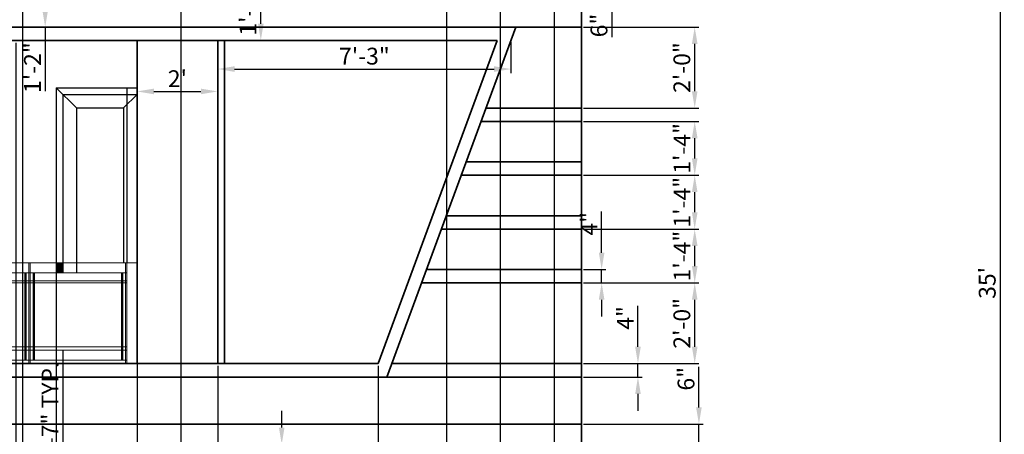
# Model space of a CAD drawing. Units: inches. Extents: x 2406 to 2953, y 1777 to 2285.
# Tile 4 of 5: x 2661 to 2953, y 1987 to 2111. Entities that reach past the tile are written whole.
import ezdxf

# ---------------------------------------------------------------- set-up
doc = ezdxf.new("R2010")
doc.units = ezdxf.units.IN
for name, color, linetype, lineweight in [('A-ANNO-DIMS', 2, 'Continuous', 18), ('A-ELEV', 7, 'Continuous', 35), ('A-ELEV-PATT', 253, 'Continuous', 13), ('A-FLOR-HRAL', 6, 'Continuous', 18), ('A-GLAZ', 4, 'Continuous', 25)]:
    doc.layers.add(name, color=color, linetype=linetype, lineweight=lineweight)
doc.styles.get("Standard").update_dxf_attribs({"font": 'arial.ttf'})
doc.dimstyles.new('ISO-25', dxfattribs={"dimtxt": 5, "dimasz": 5, "dimexe": 1.25, "dimexo": 0.625, "dimtad": 1, "dimdec": 0, "dimlunit": 3, "dimtxsty": 'Standard', "dimcen": 2.5, "dimadec": 0, "dimazin": 0, "dimtfac": 1, "dimtdec": 0, "dimtmove": 0, "dimatfit": 3, "dimfxl": 1, "dimarcsym": 0})

# ---------------------------------------------------------------- blocks, each defined once
blk = doc.blocks.new('*D1')
at = {"layer": 'A-ANNO-DIMS', "color": 0, "lineweight": -2, "transparency": 16777216}
for p, q in [((2828.46, 2242.34), (2953.44, 2242.34)), ((2952.19, 2237.34), (2952.19, 1827.34)), ((2828.46, 1822.34), (2953.44, 1822.34))]:
    blk.add_line(p, q, dxfattribs=at)
at = {"layer": 'A-ANNO-DIMS', "color": 0, "transparency": 16777216}
for points in [[(2951.35, 2237.34), (2953.02, 2237.34), (2952.19, 2242.34)], [(2951.35, 1827.34), (2953.02, 1827.34), (2952.19, 1822.34)]]:
    blk.add_solid(points, dxfattribs=at)
at = {"layer": 'Defpoints', "color": 0, "transparency": 16777216}
for p in [(2827.83, 2242.34), (2827.83, 1822.34), (2952.19, 1822.34)]:
    blk.add_point(p, dxfattribs=at)
at = {"layer": 'A-ANNO-DIMS', "color": 0, "transparency": 16777216, "insert": (2949.01, 2032.34), "char_height": 5, "attachment_point": 5, "rotation": 90}
blk.add_mtext("35'", dxfattribs=at)
blk = doc.blocks.new('*D4')
at = {"layer": 'A-ANNO-DIMS', "color": 0, "lineweight": -2, "transparency": 16777216}
for p, q in [((2719.83, 2103.72), (2719.83, 2094.64)), ((2806.9, 2103.89), (2806.9, 2094.64)), ((2724.83, 2095.89), (2801.9, 2095.89))]:
    blk.add_line(p, q, dxfattribs=at)
at = {"layer": 'A-ANNO-DIMS', "color": 0, "transparency": 16777216}
for points in [[(2724.83, 2096.72), (2724.83, 2095.05), (2719.83, 2095.89)], [(2801.9, 2096.72), (2801.9, 2095.05), (2806.9, 2095.89)]]:
    blk.add_solid(points, dxfattribs=at)
at = {"layer": 'Defpoints', "color": 0, "transparency": 16777216}
for p in [(2719.83, 2104.34), (2806.9, 2104.52), (2806.9, 2095.89)]:
    blk.add_point(p, dxfattribs=at)
at = {"layer": 'A-ANNO-DIMS', "color": 0, "transparency": 16777216, "insert": (2763.37, 2099.07), "char_height": 5, "attachment_point": 5}
blk.add_mtext('7\'-3"', dxfattribs=at)
blk = doc.blocks.new('*D19')
at = {"layer": 'A-ANNO-DIMS', "color": 0, "lineweight": -2, "transparency": 16777216}
for p, q in [((2862.73, 1995.34), (2862.73, 2007.37)), ((2828.46, 1990.34), (2863.98, 1990.34)), ((2862.73, 1984.34), (2862.73, 1990.34)), ((2828.46, 1984.34), (2863.98, 1984.34)), ((2862.73, 1979.34), (2862.73, 1974.34))]:
    blk.add_line(p, q, dxfattribs=at)
at = {"layer": 'A-ANNO-DIMS', "color": 0, "transparency": 16777216}
for points in [[(2861.89, 1995.34), (2863.56, 1995.34), (2862.73, 1990.34)], [(2861.89, 1979.34), (2863.56, 1979.34), (2862.73, 1984.34)]]:
    blk.add_solid(points, dxfattribs=at)
at = {"layer": 'Defpoints', "color": 0, "transparency": 16777216}
for p in [(2827.83, 1990.34), (2862.73, 1990.34), (2827.83, 1984.34)]:
    blk.add_point(p, dxfattribs=at)
at = {"layer": 'A-ANNO-DIMS', "color": 0, "transparency": 16777216, "insert": (2859.55, 2003.85), "char_height": 5, "attachment_point": 5, "rotation": 90}
blk.add_mtext('6"', dxfattribs=at)
blk = doc.blocks.new('*D20')
at = {"layer": 'A-ANNO-DIMS', "color": 0, "lineweight": -2, "transparency": 16777216}
for p, q in [((2844.62, 2013.34), (2844.62, 2025.54)), ((2828.46, 2008.34), (2845.87, 2008.34)), ((2844.62, 2004.34), (2844.62, 2008.34)), ((2828.46, 2004.34), (2845.87, 2004.34)), ((2844.62, 1999.34), (2844.62, 1994.34))]:
    blk.add_line(p, q, dxfattribs=at)
at = {"layer": 'A-ANNO-DIMS', "color": 0, "transparency": 16777216}
for points in [[(2843.79, 2013.34), (2845.46, 2013.34), (2844.62, 2008.34)], [(2843.79, 1999.34), (2845.46, 1999.34), (2844.62, 2004.34)]]:
    blk.add_solid(points, dxfattribs=at)
at = {"layer": 'Defpoints', "color": 0, "transparency": 16777216}
for p in [(2827.83, 2008.34), (2844.62, 2008.34), (2827.83, 2004.34)]:
    blk.add_point(p, dxfattribs=at)
at = {"layer": 'A-ANNO-DIMS', "color": 0, "transparency": 16777216, "insert": (2841.5, 2021.94), "char_height": 5, "attachment_point": 5, "rotation": 90}
blk.add_mtext('4"', dxfattribs=at)
blk = doc.blocks.new('*D21')
at = {"layer": 'A-ANNO-DIMS', "color": 0, "lineweight": -2, "transparency": 16777216}
for p, q in [((2833.84, 2041.31), (2833.84, 2053.51)), ((2828.46, 2036.31), (2835.09, 2036.31)), ((2833.84, 2032.31), (2833.84, 2036.31)), ((2828.46, 2032.31), (2835.09, 2032.31)), ((2833.84, 2027.31), (2833.84, 2022.31))]:
    blk.add_line(p, q, dxfattribs=at)
at = {"layer": 'A-ANNO-DIMS', "color": 0, "transparency": 16777216}
for points in [[(2833, 2041.31), (2834.67, 2041.31), (2833.84, 2036.31)], [(2833, 2027.31), (2834.67, 2027.31), (2833.84, 2032.31)]]:
    blk.add_solid(points, dxfattribs=at)
at = {"layer": 'Defpoints', "color": 0, "transparency": 16777216}
for p in [(2827.83, 2036.31), (2833.84, 2036.31), (2827.83, 2032.31)]:
    blk.add_point(p, dxfattribs=at)
at = {"layer": 'A-ANNO-DIMS', "color": 0, "transparency": 16777216, "insert": (2830.71, 2049.91), "char_height": 5, "attachment_point": 5, "rotation": 90}
blk.add_mtext('4"', dxfattribs=at)
blk = doc.blocks.new('*D25')
at = {"layer": 'A-ANNO-DIMS', "color": 0, "lineweight": -2, "transparency": 16777216}
for p, q in [((2695.83, 2094.79), (2695.83, 2087.98)), ((2719.83, 2095.26), (2719.83, 2087.98)), ((2700.83, 2089.23), (2714.83, 2089.23))]:
    blk.add_line(p, q, dxfattribs=at)
at = {"layer": 'A-ANNO-DIMS', "color": 0, "transparency": 16777216}
for points in [[(2700.83, 2090.06), (2700.83, 2088.4), (2695.83, 2089.23)], [(2714.83, 2090.06), (2714.83, 2088.4), (2719.83, 2089.23)]]:
    blk.add_solid(points, dxfattribs=at)
at = {"layer": 'Defpoints', "color": 0, "transparency": 16777216}
for p in [(2695.83, 2095.42), (2719.83, 2095.89), (2719.83, 2089.23)]:
    blk.add_point(p, dxfattribs=at)
at = {"layer": 'A-ANNO-DIMS', "color": 0, "transparency": 16777216, "insert": (2707.83, 2092.37), "char_height": 5, "attachment_point": 5}
blk.add_mtext("2'", dxfattribs=at)
blk = doc.blocks.new('*D26')
at = {"layer": 'A-ANNO-DIMS', "color": 0, "lineweight": -2, "transparency": 16777216}
for p, q in [((2680.71, 2122.34), (2667.31, 2122.34)), ((2668.56, 2117.34), (2668.56, 2113.34)), ((2680.71, 2108.34), (2667.31, 2108.34)), ((2668.56, 2108.34), (2668.56, 2089.27))]:
    blk.add_line(p, q, dxfattribs=at)
at = {"layer": 'A-ANNO-DIMS', "color": 0, "transparency": 16777216}
for points in [[(2667.73, 2117.34), (2669.4, 2117.34), (2668.56, 2122.34)], [(2667.73, 2113.34), (2669.4, 2113.34), (2668.56, 2108.34)]]:
    blk.add_solid(points, dxfattribs=at)
at = {"layer": 'Defpoints', "color": 0, "transparency": 16777216}
for p in [(2681.33, 2122.34), (2668.56, 2108.34), (2681.33, 2108.34)]:
    blk.add_point(p, dxfattribs=at)
at = {"layer": 'A-ANNO-DIMS', "color": 0, "transparency": 16777216, "insert": (2665.43, 2096.31), "char_height": 5, "attachment_point": 5, "rotation": 90}
blk.add_mtext('1\'-2"', dxfattribs=at)
blk = doc.blocks.new('*D27')
at = {"layer": 'A-ANNO-DIMS', "color": 0, "lineweight": -2, "transparency": 16777216}
for p, q in [((2737.53, 2122.34), (2731.35, 2122.34)), ((2732.6, 2109.34), (2732.6, 2117.34)), ((2737.53, 2104.34), (2731.35, 2104.34))]:
    blk.add_line(p, q, dxfattribs=at)
at = {"layer": 'A-ANNO-DIMS', "color": 0, "transparency": 16777216}
for points in [[(2731.77, 2117.34), (2733.44, 2117.34), (2732.6, 2122.34)], [(2731.77, 2109.34), (2733.44, 2109.34), (2732.6, 2104.34)]]:
    blk.add_solid(points, dxfattribs=at)
at = {"layer": 'Defpoints', "color": 0, "transparency": 16777216}
for p in [(2732.6, 2122.34), (2738.16, 2122.34), (2738.16, 2104.34)]:
    blk.add_point(p, dxfattribs=at)
at = {"layer": 'A-ANNO-DIMS', "color": 0, "transparency": 16777216, "insert": (2729.43, 2113.34), "char_height": 5, "attachment_point": 5, "rotation": 90}
blk.add_mtext('1\'-6"', dxfattribs=at)
blk = doc.blocks.new('*D29')
at = {"layer": 'A-ANNO-DIMS', "color": 0, "lineweight": -2, "transparency": 16777216}
for p, q in [((2836.87, 2133.34), (2836.87, 2138.34)), ((2828.46, 2128.34), (2838.12, 2128.34)), ((2836.87, 2128.34), (2836.87, 2122.34)), ((2828.46, 2122.34), (2838.12, 2122.34)), ((2836.87, 2117.34), (2836.87, 2105.32))]:
    blk.add_line(p, q, dxfattribs=at)
at = {"layer": 'A-ANNO-DIMS', "color": 0, "transparency": 16777216}
for points in [[(2836.03, 2133.34), (2837.7, 2133.34), (2836.87, 2128.34)], [(2836.03, 2117.34), (2837.7, 2117.34), (2836.87, 2122.34)]]:
    blk.add_solid(points, dxfattribs=at)
at = {"layer": 'Defpoints', "color": 0, "transparency": 16777216}
for p in [(2827.83, 2128.34), (2827.83, 2122.34), (2836.87, 2122.34)]:
    blk.add_point(p, dxfattribs=at)
at = {"layer": 'A-ANNO-DIMS', "color": 0, "transparency": 16777216, "insert": (2833.69, 2108.83), "char_height": 5, "attachment_point": 5, "rotation": 90}
blk.add_mtext('6"', dxfattribs=at)
blk = doc.blocks.new('*D32')
at = {"layer": 'A-ANNO-DIMS', "color": 0, "lineweight": -2, "transparency": 16777216}
for p, q in [((2738.81, 1989.34), (2738.81, 1994.34)), ((2748.35, 1984.34), (2737.56, 1984.34)), ((2738.81, 1975.34), (2738.81, 1984.34)), ((2748.35, 1975.34), (2737.56, 1975.34)), ((2738.81, 1970.34), (2738.81, 1965.34))]:
    blk.add_line(p, q, dxfattribs=at)
at = {"layer": 'A-ANNO-DIMS', "color": 0, "transparency": 16777216}
for points in [[(2737.98, 1989.34), (2739.65, 1989.34), (2738.81, 1984.34)], [(2737.98, 1970.34), (2739.65, 1970.34), (2738.81, 1975.34)]]:
    blk.add_solid(points, dxfattribs=at)
at = {"layer": 'Defpoints', "color": 0, "transparency": 16777216}
for p in [(2738.81, 1984.34), (2748.98, 1984.34), (2748.98, 1975.34)]:
    blk.add_point(p, dxfattribs=at)
at = {"layer": 'A-ANNO-DIMS', "color": 0, "transparency": 16777216, "insert": (2735.64, 1979.84), "char_height": 5, "attachment_point": 5, "rotation": 90}
blk.add_mtext('9"', dxfattribs=at)
blk = doc.blocks.new('*D45')
at = {"layer": 'A-ANNO-DIMS', "color": 0, "lineweight": -2, "transparency": 16777216}
for p, q in [((2673.85, 1912.9), (2673.85, 2012.41)), ((2681.47, 1912.9), (2672.6, 1912.9)), ((2673.85, 1862.91), (2673.85, 1907.9)), ((2681.47, 1857.91), (2672.6, 1857.91))]:
    blk.add_line(p, q, dxfattribs=at)
at = {"layer": 'A-ANNO-DIMS', "color": 0, "transparency": 16777216}
for points in [[(2673.01, 1907.9), (2674.68, 1907.9), (2673.85, 1912.9)], [(2673.01, 1862.91), (2674.68, 1862.91), (2673.85, 1857.91)]]:
    blk.add_solid(points, dxfattribs=at)
at = {"layer": 'Defpoints', "color": 0, "transparency": 16777216}
for p in [(2673.85, 1912.9), (2682.1, 1912.9), (2682.1, 1857.91)]:
    blk.add_point(p, dxfattribs=at)
at = {"layer": 'A-ANNO-DIMS', "color": 0, "transparency": 16777216, "insert": (2670.64, 1965.16), "char_height": 5, "attachment_point": 5, "rotation": 90}
blk.add_mtext('GATE ORNAMENT 4\'-7" TYP.', dxfattribs=at)
blk = doc.blocks.new('*D51')
at = {"layer": 'A-ANNO-DIMS', "color": 0, "lineweight": -2, "transparency": 16777216}
for p, q in [((2787.83, 1984.97), (2787.83, 2275.24)), ((2792.83, 2273.99), (2798.83, 2273.99)), ((2803.83, 1984.97), (2803.83, 2275.24))]:
    blk.add_line(p, q, dxfattribs=at)
at = {"layer": 'A-ANNO-DIMS', "color": 0, "transparency": 16777216}
for points in [[(2792.83, 2274.82), (2792.83, 2273.16), (2787.83, 2273.99)], [(2798.83, 2274.82), (2798.83, 2273.16), (2803.83, 2273.99)]]:
    blk.add_solid(points, dxfattribs=at)
at = {"layer": 'Defpoints', "color": 0, "transparency": 16777216}
for p in [(2803.83, 2273.99), (2787.83, 1984.34), (2803.83, 1984.34)]:
    blk.add_point(p, dxfattribs=at)
at = {"layer": 'A-ANNO-DIMS', "color": 0, "transparency": 16777216, "insert": (2795.83, 2277.13), "char_height": 5, "attachment_point": 5}
blk.add_mtext('1\'-4"', dxfattribs=at)
blk = doc.blocks.new('*D52')
at = {"layer": 'A-ANNO-DIMS', "color": 0, "lineweight": -2, "transparency": 16777216}
for p, q in [((2803.83, 1984.97), (2803.83, 2275.24)), ((2808.83, 2273.99), (2814.83, 2273.99)), ((2819.83, 1984.97), (2819.83, 2275.24))]:
    blk.add_line(p, q, dxfattribs=at)
at = {"layer": 'A-ANNO-DIMS', "color": 0, "transparency": 16777216}
for points in [[(2808.83, 2274.82), (2808.83, 2273.16), (2803.83, 2273.99)], [(2814.83, 2274.82), (2814.83, 2273.16), (2819.83, 2273.99)]]:
    blk.add_solid(points, dxfattribs=at)
at = {"layer": 'Defpoints', "color": 0, "transparency": 16777216}
for p in [(2819.83, 2273.99), (2803.83, 1984.34), (2819.83, 1984.34)]:
    blk.add_point(p, dxfattribs=at)
at = {"layer": 'A-ANNO-DIMS', "color": 0, "transparency": 16777216, "insert": (2811.83, 2277.13), "char_height": 5, "attachment_point": 5}
blk.add_mtext('1\'-4"', dxfattribs=at)
blk = doc.blocks.new('*D53')
at = {"layer": 'A-ANNO-DIMS', "color": 0, "lineweight": -2, "transparency": 16777216}
for p, q in [((2814.83, 2273.99), (2809.83, 2273.99)), ((2819.83, 1984.97), (2819.83, 2275.24)), ((2819.83, 2273.99), (2827.83, 2273.99)), ((2827.83, 1984.97), (2827.83, 2275.24)), ((2832.83, 2273.99), (2852.37, 2273.99))]:
    blk.add_line(p, q, dxfattribs=at)
at = {"layer": 'A-ANNO-DIMS', "color": 0, "transparency": 16777216}
for points in [[(2814.83, 2274.82), (2814.83, 2273.16), (2819.83, 2273.99)], [(2832.83, 2274.82), (2832.83, 2273.16), (2827.83, 2273.99)]]:
    blk.add_solid(points, dxfattribs=at)
at = {"layer": 'Defpoints', "color": 0, "transparency": 16777216}
for p in [(2827.83, 2273.99), (2819.83, 1984.34), (2827.83, 1984.34)]:
    blk.add_point(p, dxfattribs=at)
at = {"layer": 'A-ANNO-DIMS', "color": 0, "transparency": 16777216, "insert": (2845.1, 2277.17), "char_height": 5, "attachment_point": 5}
blk.add_mtext('0\'-8"', dxfattribs=at)
blk = doc.blocks.new('*D64')
at = {"layer": 'A-ANNO-DIMS', "color": 0, "lineweight": -2, "transparency": 16777216}
for p, q in [((2659.83, 2103.72), (2659.83, 1793.44)), ((2671.83, 2089.72), (2671.83, 1793.44)), ((2664.83, 1794.69), (2666.83, 1794.69)), ((2671.83, 1794.69), (2690.9, 1794.69))]:
    blk.add_line(p, q, dxfattribs=at)
at = {"layer": 'A-ANNO-DIMS', "color": 0, "transparency": 16777216}
for points in [[(2664.83, 1795.52), (2664.83, 1793.86), (2659.83, 1794.69)], [(2666.83, 1795.52), (2666.83, 1793.86), (2671.83, 1794.69)]]:
    blk.add_solid(points, dxfattribs=at)
at = {"layer": 'Defpoints', "color": 0, "transparency": 16777216}
for p in [(2659.83, 2104.34), (2671.83, 2090.34), (2671.83, 1794.69)]:
    blk.add_point(p, dxfattribs=at)
at = {"layer": 'A-ANNO-DIMS', "color": 0, "transparency": 16777216, "insert": (2683.87, 1797.87), "char_height": 5, "attachment_point": 5}
blk.add_mtext('1\'-0"', dxfattribs=at)
blk = doc.blocks.new('*D65')
at = {"layer": 'A-ANNO-DIMS', "color": 0, "lineweight": -2, "transparency": 16777216}
for p, q in [((2671.83, 2089.72), (2671.83, 1793.44)), ((2695.83, 2089.72), (2695.83, 1793.44)), ((2676.83, 1794.69), (2690.83, 1794.69))]:
    blk.add_line(p, q, dxfattribs=at)
at = {"layer": 'A-ANNO-DIMS', "color": 0, "transparency": 16777216}
for points in [[(2676.83, 1795.52), (2676.83, 1793.86), (2671.83, 1794.69)], [(2690.83, 1795.52), (2690.83, 1793.86), (2695.83, 1794.69)]]:
    blk.add_solid(points, dxfattribs=at)
at = {"layer": 'Defpoints', "color": 0, "transparency": 16777216}
for p in [(2671.83, 2090.34), (2695.83, 2090.34), (2695.83, 1794.69)]:
    blk.add_point(p, dxfattribs=at)
at = {"layer": 'A-ANNO-DIMS', "color": 0, "transparency": 16777216, "insert": (2683.83, 1797.87), "char_height": 5, "attachment_point": 5}
blk.add_mtext('2\'-0"', dxfattribs=at)
blk = doc.blocks.new('*D67')
at = {"layer": 'A-ANNO-DIMS', "color": 0, "lineweight": -2, "transparency": 16777216}
for p, q in [((2719.83, 2007.72), (2719.83, 1793.44)), ((2767.46, 2007.72), (2767.46, 1793.44)), ((2724.83, 1794.69), (2762.46, 1794.69))]:
    blk.add_line(p, q, dxfattribs=at)
at = {"layer": 'A-ANNO-DIMS', "color": 0, "transparency": 16777216}
for points in [[(2724.83, 1795.52), (2724.83, 1793.86), (2719.83, 1794.69)], [(2762.46, 1795.52), (2762.46, 1793.86), (2767.46, 1794.69)]]:
    blk.add_solid(points, dxfattribs=at)
at = {"layer": 'Defpoints', "color": 0, "transparency": 16777216}
for p in [(2719.83, 2008.34), (2767.46, 2008.34), (2767.46, 1794.69)]:
    blk.add_point(p, dxfattribs=at)
at = {"layer": 'A-ANNO-DIMS', "color": 0, "transparency": 16777216, "insert": (2743.65, 1797.9), "char_height": 5, "attachment_point": 5}
blk.add_mtext('3\'-11 1/2"', dxfattribs=at)
blk = doc.blocks.new('*D68')
at = {"layer": 'A-ANNO-DIMS', "color": 0, "lineweight": -2, "transparency": 16777216}
for p, q in [((2828.46, 2032.31), (2862.73, 2032.31)), ((2861.48, 2013.34), (2861.48, 2027.31)), ((2828.46, 2008.34), (2862.73, 2008.34))]:
    blk.add_line(p, q, dxfattribs=at)
at = {"layer": 'A-ANNO-DIMS', "color": 0, "transparency": 16777216}
for points in [[(2860.65, 2027.31), (2862.32, 2027.31), (2861.48, 2032.31)], [(2860.65, 2013.34), (2862.32, 2013.34), (2861.48, 2008.34)]]:
    blk.add_solid(points, dxfattribs=at)
at = {"layer": 'Defpoints', "color": 0, "transparency": 16777216}
for p in [(2827.83, 2032.31), (2861.48, 2032.31), (2827.83, 2008.34)]:
    blk.add_point(p, dxfattribs=at)
at = {"layer": 'A-ANNO-DIMS', "color": 0, "transparency": 16777216, "insert": (2858.31, 2020.32), "char_height": 5, "attachment_point": 5, "rotation": 90}
blk.add_mtext('2\'-0"', dxfattribs=at)
blk = doc.blocks.new('*D69')
at = {"layer": 'A-ANNO-DIMS', "color": 0, "lineweight": -2, "transparency": 16777216}
for p, q in [((2828.46, 2048.31), (2862.73, 2048.31)), ((2861.48, 2037.31), (2861.48, 2043.31)), ((2828.46, 2032.31), (2862.73, 2032.31))]:
    blk.add_line(p, q, dxfattribs=at)
at = {"layer": 'A-ANNO-DIMS', "color": 0, "transparency": 16777216}
for points in [[(2860.65, 2043.31), (2862.32, 2043.31), (2861.48, 2048.31)], [(2860.65, 2037.31), (2862.32, 2037.31), (2861.48, 2032.31)]]:
    blk.add_solid(points, dxfattribs=at)
at = {"layer": 'Defpoints', "color": 0, "transparency": 16777216}
for p in [(2827.83, 2048.31), (2861.48, 2048.31), (2827.83, 2032.31)]:
    blk.add_point(p, dxfattribs=at)
at = {"layer": 'A-ANNO-DIMS', "color": 0, "transparency": 16777216, "insert": (2858.35, 2040.31), "char_height": 5, "attachment_point": 5, "rotation": 90}
blk.add_mtext('1\'-4"', dxfattribs=at)
blk = doc.blocks.new('*D70')
at = {"layer": 'A-ANNO-DIMS', "color": 0, "lineweight": -2, "transparency": 16777216}
for p, q in [((2828.46, 2064.31), (2862.73, 2064.31)), ((2861.48, 2053.31), (2861.48, 2059.31)), ((2828.46, 2048.31), (2862.73, 2048.31))]:
    blk.add_line(p, q, dxfattribs=at)
at = {"layer": 'A-ANNO-DIMS', "color": 0, "transparency": 16777216}
for points in [[(2860.65, 2059.31), (2862.32, 2059.31), (2861.48, 2064.31)], [(2860.65, 2053.31), (2862.32, 2053.31), (2861.48, 2048.31)]]:
    blk.add_solid(points, dxfattribs=at)
at = {"layer": 'Defpoints', "color": 0, "transparency": 16777216}
for p in [(2827.83, 2064.31), (2861.48, 2064.31), (2827.83, 2048.31)]:
    blk.add_point(p, dxfattribs=at)
at = {"layer": 'A-ANNO-DIMS', "color": 0, "transparency": 16777216, "insert": (2858.35, 2056.31), "char_height": 5, "attachment_point": 5, "rotation": 90}
blk.add_mtext('1\'-4"', dxfattribs=at)
blk = doc.blocks.new('*D71')
at = {"layer": 'A-ANNO-DIMS', "color": 0, "lineweight": -2, "transparency": 16777216}
for p, q in [((2828.46, 2080.31), (2862.73, 2080.31)), ((2861.48, 2069.31), (2861.48, 2075.31)), ((2828.46, 2064.31), (2862.73, 2064.31))]:
    blk.add_line(p, q, dxfattribs=at)
at = {"layer": 'A-ANNO-DIMS', "color": 0, "transparency": 16777216}
for points in [[(2860.65, 2075.31), (2862.32, 2075.31), (2861.48, 2080.31)], [(2860.65, 2069.31), (2862.32, 2069.31), (2861.48, 2064.31)]]:
    blk.add_solid(points, dxfattribs=at)
at = {"layer": 'Defpoints', "color": 0, "transparency": 16777216}
for p in [(2827.83, 2080.31), (2861.48, 2080.31), (2827.83, 2064.31)]:
    blk.add_point(p, dxfattribs=at)
at = {"layer": 'A-ANNO-DIMS', "color": 0, "transparency": 16777216, "insert": (2858.35, 2072.31), "char_height": 5, "attachment_point": 5, "rotation": 90}
blk.add_mtext('1\'-4"', dxfattribs=at)
blk = doc.blocks.new('*D72')
at = {"layer": 'A-ANNO-DIMS', "color": 0, "lineweight": -2, "transparency": 16777216}
for p, q in [((2828.46, 2108.34), (2862.73, 2108.34)), ((2861.48, 2089.31), (2861.48, 2103.34)), ((2828.46, 2084.31), (2862.73, 2084.31))]:
    blk.add_line(p, q, dxfattribs=at)
at = {"layer": 'A-ANNO-DIMS', "color": 0, "transparency": 16777216}
for points in [[(2860.65, 2103.34), (2862.32, 2103.34), (2861.48, 2108.34)], [(2860.65, 2089.31), (2862.32, 2089.31), (2861.48, 2084.31)]]:
    blk.add_solid(points, dxfattribs=at)
at = {"layer": 'Defpoints', "color": 0, "transparency": 16777216}
for p in [(2827.83, 2108.34), (2861.48, 2108.34), (2827.83, 2084.31)]:
    blk.add_point(p, dxfattribs=at)
at = {"layer": 'A-ANNO-DIMS', "color": 0, "transparency": 16777216, "insert": (2858.31, 2096.32), "char_height": 5, "attachment_point": 5, "rotation": 90}
blk.add_mtext('2\'-0"', dxfattribs=at)
blk = doc.blocks.new('*D82')
at = {"layer": 'A-ANNO-DIMS', "color": 0, "lineweight": -2, "transparency": 16777216}
for p, q in [((2661.83, 2155.72), (2661.83, 1793.44)), ((2708.83, 2155.72), (2708.83, 1793.44)), ((2666.83, 1794.69), (2703.83, 1794.69))]:
    blk.add_line(p, q, dxfattribs=at)
at = {"layer": 'A-ANNO-DIMS', "color": 0, "transparency": 16777216}
for points in [[(2666.83, 1795.52), (2666.83, 1793.86), (2661.83, 1794.69)], [(2703.83, 1795.52), (2703.83, 1793.86), (2708.83, 1794.69)]]:
    blk.add_solid(points, dxfattribs=at)
at = {"layer": 'Defpoints', "color": 0, "transparency": 16777216}
for p in [(2661.83, 2156.34), (2708.83, 2156.34), (2708.83, 1794.69)]:
    blk.add_point(p, dxfattribs=at)
at = {"layer": 'A-ANNO-DIMS', "color": 0, "transparency": 16777216, "insert": (2685.33, 1797.87), "char_height": 5, "attachment_point": 5}
blk.add_mtext('3\'-11"', dxfattribs=at)

msp = doc.modelspace()

# ---------------------------------------------------------------- hatches: boundary and pattern name
at = {"layer": 'A-ELEV-PATT'}
h = msp.add_hatch(color=256, dxfattribs=at)
h.dxf.hatch_style = 1
h.paths.add_polyline_path([(2671.83, 2038.34), (2671.83, 2035.34), (2673.83, 2035.34), (2673.83, 2038.34)])

# ---------------------------------------------------------------- linework, layer by layer
at = {"layer": 'A-ELEV'}
for p, q in [((2827.83, 1822.34), (2827.83, 2167.34)), ((2463.83, 2108.34), (2827.83, 2108.34)), ((2808.31, 2108.34), (2769.99, 2004.34)), ((2467.83, 2104.34), (2802.83, 2104.34)), ((2695.83, 2038.34), (2695.83, 2104.34)), ((2719.83, 2008.34), (2719.83, 2104.34)), ((2721.83, 2008.34), (2721.83, 2104.34)), ((2802.83, 2104.34), (2767.46, 2008.34)), ((2695.83, 2090.34), (2695.83, 2008.34)), ((2799.45, 2084.31), (2827.83, 2084.31)), ((2797.98, 2080.31), (2827.83, 2080.31)), ((2793.56, 2068.31), (2827.83, 2068.31)), ((2792.08, 2064.31), (2827.83, 2064.31)), ((2787.66, 2052.31), (2827.83, 2052.31)), ((2786.19, 2048.31), (2827.83, 2048.31)), ((2781.77, 2036.31), (2827.83, 2036.31)), ((2780.29, 2032.31), (2827.83, 2032.31)), ((2467.83, 2008.34), (2767.46, 2008.34)), ((2771.46, 2008.34), (2827.83, 2008.34)), ((2463.83, 2004.34), (2827.83, 2004.34)), ((2443.83, 1990.34), (2827.83, 1990.34))]:
    msp.add_line(p, q, dxfattribs=at)
at = {"layer": 'A-FLOR-HRAL'}
for p, q in [((2467.83, 2038.34), (2695.83, 2038.34)), ((2663.74, 2038.34), (2663.74, 2008.34)), ((2664.14, 2038.34), (2664.14, 2008.34)), ((2692.41, 2038.34), (2692.41, 2008.34)), ((2692.81, 2038.34), (2692.81, 2008.34)), ((2469.83, 2035.34), (2692.83, 2035.34)), ((2662.54, 2035.34), (2662.54, 2009.34)), ((2662.74, 2035.34), (2662.74, 2009.34)), ((2662.94, 2035.34), (2662.94, 2009.34)), ((2664.94, 2035.34), (2664.94, 2009.34)), ((2665.14, 2035.34), (2665.14, 2009.34)), ((2665.34, 2035.34), (2665.34, 2009.34)), ((2691.21, 2035.34), (2691.21, 2009.34)), ((2691.41, 2035.34), (2691.41, 2009.34)), ((2691.61, 2035.34), (2691.61, 2009.34)), ((2692.83, 2035.34), (2692.83, 2009.34)), ((2469.83, 2009.34), (2692.83, 2009.34))]:
    msp.add_line(p, q, dxfattribs=at)
for points in [[(2468.63, 2032.98), (2692.83, 2032.98), (2692.83, 2032.31), (2468.63, 2032.31)], [(2468.63, 2013.35), (2692.83, 2013.35), (2692.83, 2012.3), (2468.63, 2012.3)]]:
    msp.add_lwpolyline(points, close=True, dxfattribs=at)
at = {"layer": 'A-GLAZ'}
for p, q in [((2671.83, 2090.34), (2695.83, 2090.34)), ((2671.83, 2090.34), (2671.83, 2035.34)), ((2677.83, 2084.34), (2671.83, 2090.34)), ((2673.83, 2088.34), (2673.83, 2035.34)), ((2673.83, 2088.34), (2695.83, 2088.34)), ((2691.83, 2084.34), (2695.83, 2088.34)), ((2692.83, 2090.34), (2692.83, 2038.34)), ((2677.83, 2084.34), (2691.83, 2084.34)), ((2677.83, 2084.34), (2677.83, 2035.34)), ((2691.83, 2084.34), (2691.83, 2038.34))]:
    msp.add_line(p, q, dxfattribs=at)

# ---------------------------------------------------------------- dimensions: what is measured, and where the dimension line sits
at = {"layer": 'A-ANNO-DIMS'}
for base, p1, p2, override, picture, middle in [((2803.83, 2273.99), (2787.83, 1984.34), (2803.83, 1984.34), {"dimdec": 1, "dimlfac": 1, "dimrnd": 0, "dimzin": 1, "dimdsep": 46, "dimlunit": 4, "dimfrac": 2}, '*D51', (2795.83, 2277.13)), ((2819.83, 2273.99), (2803.83, 1984.34), (2819.83, 1984.34), {"dimdec": 1, "dimlfac": 1, "dimrnd": 0, "dimzin": 1, "dimdsep": 46, "dimlunit": 4, "dimfrac": 2}, '*D52', (2811.83, 2277.13)), ((2827.83, 2273.99), (2819.83, 1984.34), (2827.83, 1984.34), {"dimdec": 1, "dimlfac": 1, "dimrnd": 0, "dimzin": 1, "dimdsep": 46, "dimlunit": 4, "dimfrac": 2}, '*D53', (2845.1, 2277.17)), ((2708.83, 1794.69), (2661.83, 2156.34), (2708.83, 2156.34), {"dimdec": 1, "dimlfac": 1, "dimrnd": 0, "dimzin": 1, "dimdsep": 46, "dimlunit": 4, "dimfrac": 2}, '*D82', (2685.33, 1797.87)), ((2671.83, 1794.69), (2659.83, 2104.34), (2671.83, 2090.34), {"dimdec": 1, "dimlfac": 1, "dimrnd": 0, "dimzin": 1, "dimdsep": 46, "dimlunit": 4, "dimfrac": 2}, '*D64', (2683.87, 1797.87)), ((2806.9, 2095.89), (2719.83, 2104.34), (2806.9, 2104.52), {"dimclrd": 0, "dimclre": 0, "dimclrt": 0}, '*D4', (2763.37, 2099.07)), ((2719.83, 2089.23), (2695.83, 2095.42), (2719.83, 2095.89), {"dimclrd": 0, "dimclre": 0, "dimclrt": 0}, '*D25', (2707.83, 2092.37)), ((2695.83, 1794.69), (2671.83, 2090.34), (2695.83, 2090.34), {"dimdec": 1, "dimlfac": 1, "dimrnd": 0, "dimzin": 1, "dimdsep": 46, "dimlunit": 4, "dimfrac": 2}, '*D65', (2683.83, 1797.87)), ((2767.46, 1794.69), (2719.83, 2008.34), (2767.46, 2008.34), {"dimdec": 1, "dimlfac": 1, "dimrnd": 0, "dimzin": 1, "dimdsep": 46, "dimlunit": 4, "dimfrac": 2}, '*D67', (2743.65, 1797.9))]:
    dim = msp.add_linear_dim(base=base, p1=p1, p2=p2, dimstyle='ISO-25', override=override, dxfattribs=at)
    dim.commit()
    dim.dimension.update_dxf_attribs({"geometry": picture, "text_midpoint": middle})
for base, p1, p2, override, picture, middle in [((2952.19, 1822.34), (2827.83, 2242.34), (2827.83, 1822.34), {"dimclrd": 0, "dimclre": 0, "dimclrt": 0}, '*D1', (2949.01, 2032.34)), ((2836.87, 2122.34), (2827.83, 2128.34), (2827.83, 2122.34), {"dimclrd": 0, "dimclre": 0, "dimclrt": 0}, '*D29', (2833.69, 2108.83)), ((2668.56, 2108.34), (2681.33, 2122.34), (2681.33, 2108.34), {"dimclrd": 0, "dimclre": 0, "dimclrt": 0}, '*D26', (2665.43, 2096.31)), ((2732.6, 2122.34), (2738.16, 2104.34), (2738.16, 2122.34), {"dimclrd": 0, "dimclre": 0, "dimclrt": 0}, '*D27', (2729.43, 2113.34)), ((2861.48, 2108.34), (2827.83, 2084.31), (2827.83, 2108.34), {"dimdec": 1, "dimlfac": 1, "dimrnd": 0, "dimzin": 1, "dimdsep": 46, "dimlunit": 4, "dimfrac": 2}, '*D72', (2858.31, 2096.32)), ((2861.48, 2080.31), (2827.83, 2064.31), (2827.83, 2080.31), {"dimdec": 1, "dimlfac": 1, "dimrnd": 0, "dimzin": 1, "dimdsep": 46, "dimlunit": 4, "dimfrac": 2}, '*D71', (2858.35, 2072.31)), ((2861.48, 2064.31), (2827.83, 2048.31), (2827.83, 2064.31), {"dimdec": 1, "dimlfac": 1, "dimrnd": 0, "dimzin": 1, "dimdsep": 46, "dimlunit": 4, "dimfrac": 2}, '*D70', (2858.35, 2056.31)), ((2833.84, 2036.31), (2827.83, 2032.31), (2827.83, 2036.31), {"dimclrd": 0, "dimclre": 0, "dimclrt": 0}, '*D21', (2830.71, 2049.91)), ((2861.48, 2048.31), (2827.83, 2032.31), (2827.83, 2048.31), {"dimdec": 1, "dimlfac": 1, "dimrnd": 0, "dimzin": 1, "dimdsep": 46, "dimlunit": 4, "dimfrac": 2}, '*D69', (2858.35, 2040.31)), ((2861.48, 2032.31), (2827.83, 2008.34), (2827.83, 2032.31), {"dimdec": 1, "dimlfac": 1, "dimrnd": 0, "dimzin": 1, "dimdsep": 46, "dimlunit": 4, "dimfrac": 2}, '*D68', (2858.31, 2020.32)), ((2844.62, 2008.34), (2827.83, 2004.34), (2827.83, 2008.34), {"dimclrd": 0, "dimclre": 0, "dimclrt": 0}, '*D20', (2841.5, 2021.94)), ((2862.73, 1990.34), (2827.83, 1984.34), (2827.83, 1990.34), {"dimclrd": 0, "dimclre": 0, "dimclrt": 0}, '*D19', (2859.55, 2003.85)), ((2738.81, 1984.34), (2748.98, 1975.34), (2748.98, 1984.34), {"dimclrd": 0, "dimclre": 0, "dimclrt": 0}, '*D32', (2735.64, 1979.84))]:
    dim = msp.add_linear_dim(base=base, p1=p1, p2=p2, angle=90, dimstyle='ISO-25', override=override, dxfattribs=at)
    dim.commit()
    dim.dimension.update_dxf_attribs({"geometry": picture, "text_midpoint": middle})
dim = msp.add_linear_dim(base=(2673.85, 1912.9), p1=(2682.1, 1857.91), p2=(2682.1, 1912.9), angle=90, text='GATE ORNAMENT <> TYP.', dimstyle='ISO-25', override={"dimdec": 1, "dimrnd": 0, "dimzin": 1, "dimlunit": 4, "dimfrac": 2}, dxfattribs=at)
dim.commit()
dim.dimension.update_dxf_attribs({"geometry": '*D45', "text_midpoint": (2670.64, 1965.16)})

doc.saveas('drawing.dxf')
